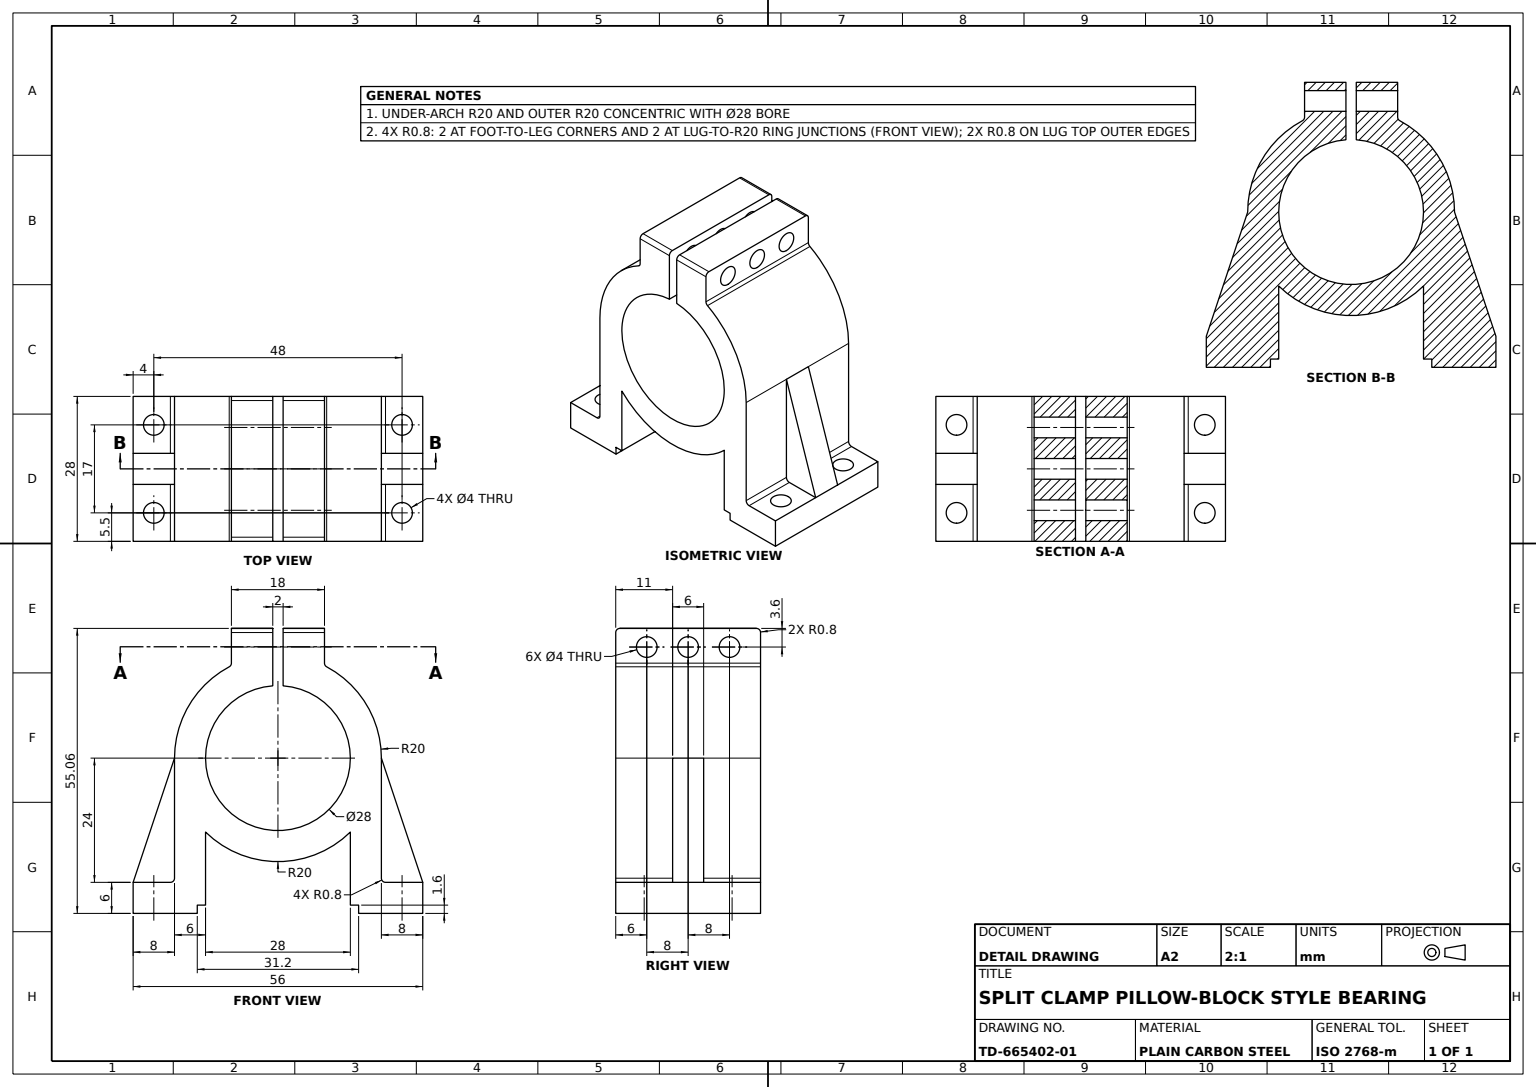
from build123d import *

# Parameters (mm, degrees)
OMEGA_PROFILE_SKETCH_R         = 14
OMEGA_BODY_DEPTH               = 28
SUPPORT_RIB_REACH              = 45.359
SUPPORT_RIB_SKETCH_WALL_W      = 114.016154836
SUPPORT_RIB_SKETCH_WALL_H      = 6
BASE_MOUNTING_HOLES_SKETCH_R   = 2
BASE_MOUNTING_HOLES_DEPTH      = 28
CLAMP_LUG_DEPTH                = 28
SPLIT_SLOT_SKETCH_W            = 2
SPLIT_SLOT_SKETCH_H            = 18.147677211
SPLIT_SLOT_2MM_DEPTH           = 28
CLAMP_SCREW_HOLES_SKETCH_R     = 2
CLAMP_SCREW_HOLES_3X_3_6_DEPTH = 28
EDGE_FILLETS_R0_8_R            = 0.8


with BuildPart() as part:
    # Omega Profile Sketch → Omega Body (new body)
    with BuildSketch(Plane.XY):
        with BuildLine():
            Line((-20, 0), (-20, -24))
            Line((-20, -24), (-28, -24))
            Line((-28, -24), (-28, -30))
            Line((-28, -30), (-15.6, -30))
            Line((-15.6, -30), (-15.6, -28.4))
            Line((-15.6, -28.4), (-14, -28.4))
            Line((-14, -28.4), (-14, -14.282856857))
            ThreePointArc((-14, -14.282856857), (0, -20), (14, -14.282856857))
            Line((14, -14.282856857), (14, -28.4))
            Line((14, -28.4), (15.6, -28.4))
            Line((15.6, -28.4), (15.6, -30))
            Line((15.6, -30), (28, -30))
            Line((28, -30), (28, -24))
            Line((28, -24), (20, -24))
            Line((20, -24), (20, 0))
            ThreePointArc((20, 0), (0, 20), (-20, 0))
        make_face()
        Circle(OMEGA_PROFILE_SKETCH_R, mode=Mode.SUBTRACT)
    extrude(amount=-OMEGA_BODY_DEPTH)

    # Support Rib Sketch wall → Support Rib (add, up to next)
    with BuildSketch(Plane(origin=(24, -12, -14), x_dir=(0.316227766017, -0.948683298051, 0), z_dir=(0.948683298051, 0.316227766017, 0)), mode=Mode.PRIVATE) as support_rib_sk1:
        Rectangle(SUPPORT_RIB_SKETCH_WALL_W, SUPPORT_RIB_SKETCH_WALL_H)
    support_rib_tool1 = extrude(support_rib_sk1.sketch, amount=-SUPPORT_RIB_REACH, mode=Mode.PRIVATE) - part.part
    support_rib = support_rib_tool1.solids().sort_by_distance((24, -12, -14))[0]
    add(support_rib)

    # Support Rib Mirror: Support Rib across plane
    add(support_rib.mirror(Plane(origin=(0, 0, 0), x_dir=(0, 0, 1), z_dir=(1, 0, 0))))

    # Base Mounting Holes Sketch → Base Mounting Holes (cut)
    with BuildSketch(Plane(origin=(0, -24, 0), x_dir=(1, 0, 0), z_dir=(0, 1, 0))):
        with Locations(Location((24, 22.5, 0), (0, 0, 270))):
            Circle(BASE_MOUNTING_HOLES_SKETCH_R)
        with Locations(Location((24, 5.5, 0), (0, 0, 270))):
            Circle(BASE_MOUNTING_HOLES_SKETCH_R)
        with Locations(Location((-24, 5.5, 0), (0, 0, 270))):
            Circle(BASE_MOUNTING_HOLES_SKETCH_R)
        with Locations(Location((-24, 22.5, 0), (0, 0, 270))):
            Circle(BASE_MOUNTING_HOLES_SKETCH_R)
    extrude(amount=-BASE_MOUNTING_HOLES_DEPTH, mode=Mode.SUBTRACT)

    # Clamp Lug Sketch → Clamp Lug (add)
    with BuildSketch(Plane.XY):
        with BuildLine():
            Line((-9, 17.860571099), (-9, 25.060571099))
            Line((-9, 25.060571099), (9, 25.060571099))
            Line((9, 25.060571099), (9, 17.860571099))
            ThreePointArc((9, 17.860571099), (0, 20), (-9, 17.860571099))
        make_face()
    extrude(amount=-CLAMP_LUG_DEPTH)

    # Split Slot Sketch → Split Slot 2mm (cut)
    with BuildSketch(Plane.XY):
        with Locations((0, 20.958575759)):
            Rectangle(SPLIT_SLOT_SKETCH_W, SPLIT_SLOT_SKETCH_H)
    extrude(amount=-SPLIT_SLOT_2MM_DEPTH, mode=Mode.SUBTRACT)

    # Clamp Screw Holes Sketch → Clamp Screw Holes 3xØ3.6 (cut)
    with BuildSketch(Plane(origin=(9, 0, 0), x_dir=(0, 0, -1), z_dir=(1, 0, 0))):
        with Locations(Location((6, 21.460571099, 0), (0, 0, 180))):
            Circle(CLAMP_SCREW_HOLES_SKETCH_R)
        with Locations(Location((14, 21.460571099, 0), (0, 0, 180))):
            Circle(CLAMP_SCREW_HOLES_SKETCH_R)
        with Locations(Location((22, 21.460571099, 0), (0, 0, 180))):
            Circle(CLAMP_SCREW_HOLES_SKETCH_R)
    extrude(amount=-CLAMP_SCREW_HOLES_3X_3_6_DEPTH, mode=Mode.SUBTRACT)

    # Edge Fillets R0.8
    edge_fillets_r0_8_edges = [part.edges().sort_by_distance(p)[0] for p in [
        (-20, -24, -5.5),
        (9, 17.860571099, -14),
        (-9, 17.860571099, -14),
        (5, 25.060571099, -28),
        (5, 25.060571099, 0),
        (-5, 25.060571099, 0),
        (-5, 25.060571099, -28),
        (20, -24, -22.5),
        (-20, -24, -22.5),
        (20, -24, -5.5),
    ]]
    fillet(edge_fillets_r0_8_edges, radius=EDGE_FILLETS_R0_8_R)


solid = part.part
